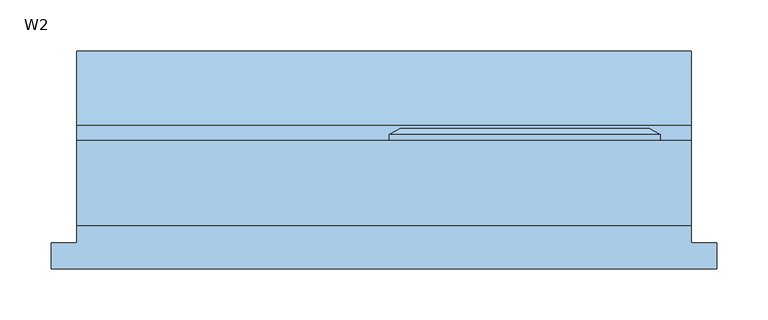
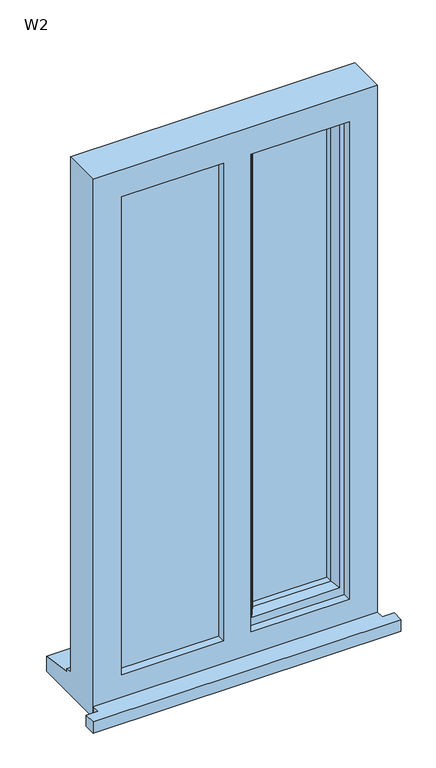
"""IFC4 building model written with IfcOpenShell, lengths in millimetres: window geometry, W2."""

from ifc_helpers import new_model, si_unit, frame, origin, place, context, project, spatial, polyline, outline, extrude, faceted_brep, source, transform, mapped, element, save


def w2_3d16f0f7(model_context):
    return source(origin(), model_context, "Body", "SolidModel", [
        extrude(outline(polyline([(-610.0, -91.5434322), (-610.0, -66.5434322), (-585.0, -66.5434322), (-585.0, -49.5434322), (15.0, -49.5434322), (15.0, -66.5434322), (40.0, -66.5434322), (40.0, -91.5434322), (-610.0, -91.5434322)])), frame((0.0, 0.0, 1200.0), z_axis=(0.0, 0.0, 1.0), x_axis=(1.0, 0.0, 0.0)), (0.0, 0.0, 1.0), 25.0),
        faceted_brep([(-280.0, 33.4565678, 2370.0), (-280.0, 39.2300705, 2370.0), (-280.0, 39.2300705, 1253.0), (-280.0, 33.4565678, 1253.0), (-270.0, -31.5434322, 2360.0), (-270.0, 33.4565678, 2360.0), (-270.0, 33.4565678, 1263.0), (-270.0, -31.5434322, 1263.0), (-230.0, -17.0505323, 2320.0), (-240.1480377, -31.5434322, 2330.1480377), (-240.1480377, -31.5434322, 1292.8519623), (-230.0, -17.0505323, 1303.0), (-230.0, -2.5434322, 2320.0), (-230.0, -2.5434322, 1303.0), (-240.0, 21.4565678, 2330.0), (-240.0, -2.5434322, 2330.0), (-240.0, -2.5434322, 1293.0), (-240.0, 21.4565678, 1293.0), (-230.0, 39.2300705, 2320.0), (-230.0, 21.4565678, 2320.0), (-230.0, 21.4565678, 1303.0), (-230.0, 39.2300705, 1303.0), (-247.4457548, 45.0035732, 2337.4457548), (-247.4457548, 45.0035732, 1285.5542452), (-269.2153903, 45.0035732, 2359.2153903), (-269.2153903, 45.0035732, 1263.7846097), (-15.0, 39.2300705, 1253.0), (-15.0, 33.4565678, 1253.0), (-25.0, 33.4565678, 1263.0), (-25.0, -31.5434322, 1263.0), (-54.8519623, -31.5434322, 1292.8519623), (-65.0, -17.0505323, 1303.0), (-65.0, -2.5434322, 1303.0), (-55.0, -2.5434322, 1293.0), (-55.0, 21.4565678, 1293.0), (-65.0, 21.4565678, 1303.0), (-65.0, 39.2300705, 1303.0), (-47.5542452, 45.0035732, 1285.5542452), (-25.7846097, 45.0035732, 1263.7846097), (-15.0, 39.2300705, 2370.0), (-15.0, 33.4565678, 2370.0), (-25.0, 33.4565678, 2360.0), (-25.0, -31.5434322, 2360.0), (-54.8519623, -31.5434322, 2330.1480377), (-65.0, -17.0505323, 2320.0), (-65.0, -2.5434322, 2320.0), (-55.0, -2.5434322, 2330.0), (-55.0, 21.4565678, 2330.0), (-65.0, 21.4565678, 2320.0), (-65.0, 39.2300705, 2320.0), (-47.5542452, 45.0035732, 2337.4457548), (-25.7846097, 45.0035732, 2359.2153903)], [[[0, 1, 2, 3]], [[4, 5, 6, 7]], [[8, 9, 10, 11]], [[12, 8, 11, 13]], [[14, 15, 16, 17]], [[18, 19, 20, 21]], [[22, 18, 21, 23]], [[1, 24, 25, 2]], [[3, 2, 26, 27]], [[7, 6, 28, 29]], [[11, 10, 30, 31]], [[13, 11, 31, 32]], [[17, 16, 33, 34]], [[21, 20, 35, 36]], [[23, 21, 36, 37]], [[2, 25, 38, 26]], [[27, 26, 39, 40]], [[29, 28, 41, 42]], [[31, 30, 43, 44]], [[32, 31, 44, 45]], [[34, 33, 46, 47]], [[36, 35, 48, 49]], [[37, 36, 49, 50]], [[26, 38, 51, 39]], [[40, 39, 1, 0]], [[3, 27, 40, 0], [5, 41, 28, 6]], [[42, 41, 5, 4]], [[7, 29, 42, 4], [9, 43, 30, 10]], [[44, 43, 9, 8]], [[45, 44, 8, 12]], [[15, 46, 33, 16], [13, 32, 45, 12]], [[47, 46, 15, 14]], [[17, 34, 47, 14], [19, 48, 35, 20]], [[49, 48, 19, 18]], [[50, 49, 18, 22]], [[24, 51, 38, 25], [23, 37, 50, 22]], [[39, 51, 24, 1]]]),
        extrude(outline(polyline([(2340.0, -310.0), (2360.0, -310.0), (2360.0, -545.0), (1263.0, -545.0), (1263.0, -310.0), (1283.0, -310.0), (1283.0, -525.0), (2340.0, -525.0), (2340.0, -310.0)])), frame((0.0, -7.5434322, 0.0), z_axis=(0.0, 1.0, 0.0), x_axis=(0.0, 0.0, 1.0)), (0.0, 0.0, 1.0), 41.0),
        faceted_brep([(15.0, -49.5434322, 2400.0), (-585.0, -49.5434322, 2400.0), (-585.0, -49.5434322, 1200.0), (15.0, -49.5434322, 1200.0), (-45.0, -49.5434322, 2340.0), (-45.0, -49.5434322, 1275.0), (-252.0, -49.5434322, 1275.0), (-252.0, -49.5434322, 2340.0), (-310.0, -49.5434322, 2340.0), (-310.0, -49.5434322, 1275.0), (-525.0, -49.5434322, 1275.0), (-525.0, -49.5434322, 2340.0), (-585.0, 33.4565678, 2400.0), (-585.0, 33.4565678, 1251.0), (-585.0, 48.4565678, 1249.68767), (-585.0, 48.4565678, 1244.7449676), (-585.0, 120.9565678, 1233.8088847), (-585.0, 120.9565678, 1200.0), (15.0, 33.4565678, 2400.0), (15.0, 33.4565678, 1251.0), (-545.0, 33.4565678, 2360.0), (-545.0, 33.4565678, 1263.0), (-310.0, 33.4565678, 1263.0), (-310.0, 33.4565678, 2360.0), (-270.0, 33.4565678, 2360.0), (-270.0, 33.4565678, 1263.0), (-25.0, 33.4565678, 1263.0), (-25.0, 33.4565678, 2360.0), (-545.0, -31.5434322, 2360.0), (-545.0, -31.5434322, 1263.0), (-300.0, -31.5434322, 2360.0), (-300.0, -31.5434322, 1263.0), (-310.0, -31.5434322, 2340.0), (-525.0, -31.5434322, 2340.0), (-525.0, -31.5434322, 1275.0), (-310.0, -31.5434322, 1275.0), (-270.0, -31.5434322, 2360.0), (-25.0, -31.5434322, 2360.0), (-25.0, -31.5434322, 1263.0), (-270.0, -31.5434322, 1263.0), (-45.0, -31.5434322, 2340.0), (-252.0, -31.5434322, 2340.0), (-252.0, -31.5434322, 1275.0), (-45.0, -31.5434322, 1275.0), (-310.0, -7.5434322, 2360.0), (-300.0, -7.5434322, 2360.0), (15.0, 120.9565678, 1200.0), (15.0, 120.9565678, 1233.8088847), (15.0, 48.4565678, 1244.7449676), (15.0, 48.4565678, 1249.68767), (-300.0, -7.5434322, 1263.0), (-310.0, -7.5434322, 1263.0)], [[[0, 1, 2, 3], [4, 5, 6, 7], [8, 9, 10, 11]], [[2, 1, 12, 13, 14, 15, 16, 17]], [[13, 12, 18, 19], [20, 21, 22, 23], [24, 25, 26, 27]], [[21, 20, 28, 29]], [[28, 30, 31, 29], [32, 33, 34, 35]], [[36, 37, 38, 39], [40, 41, 42, 43]], [[33, 11, 10, 34]], [[1, 0, 18, 12]], [[28, 20, 23, 44, 45, 30]], [[27, 37, 36, 24]], [[11, 33, 32, 8]], [[40, 4, 7, 41]], [[19, 18, 0, 3, 46, 47, 48, 49]], [[27, 26, 38, 37]], [[4, 40, 43, 5]], [[45, 50, 31, 30]], [[50, 45, 44, 51]], [[51, 44, 23, 22]], [[25, 24, 36, 39]], [[41, 7, 6, 42]], [[8, 32, 35, 9]], [[46, 3, 2, 17]], [[47, 46, 17, 16]], [[48, 47, 16, 15]], [[49, 48, 15, 14]], [[19, 49, 14, 13]], [[22, 21, 29, 31, 50, 51]], [[26, 25, 39, 38]], [[6, 5, 43, 42]], [[35, 34, 10, 9]]]),
        extrude(outline(polyline([(-545.0, -7.5434322), (-300.0, -7.5434322), (-300.0, -31.5434322), (-545.0, -31.5434322), (-545.0, -7.5434322)])), frame((0.0, 0.0, 1263.0), z_axis=(0.0, 0.0, 1.0), x_axis=(1.0, 0.0, 0.0)), (0.0, 0.0, 1.0), 1097.0),
        extrude(outline(polyline([(-55.0, -2.5434322), (-240.0, -2.5434322), (-240.0, 21.4565678), (-55.0, 21.4565678), (-55.0, -2.5434322)])), frame((0.0, 0.0, 1293.0), z_axis=(0.0, 0.0, 1.0), x_axis=(1.0, 0.0, 0.0)), (0.0, 0.0, 1.0), 1037.0),
    ])


if __name__ == "__main__":
    model = new_model("IFC4")
    model_context = context("Model", 3, world=origin())
    ifc_project = project(units=[si_unit("LENGTHUNIT", "METRE", prefix="MILLI")], contexts=[model_context])
    site = spatial("IfcSite", under=ifc_project)
    building = spatial("IfcBuilding", under=site)
    placement = place(None, origin())
    w2_shape = w2_3d16f0f7(model_context)
    element("IfcWindow", 1, ObjectType="W2", at=placement, inside=building, context=model_context, shape_type="MappedRepresentation", body=[
        mapped(w2_shape, transform((0.0, 0.0, 0.0), x_axis=(1.0, 0.0, 0.0), y_axis=(0.0, 1.0, 0.0), z_axis=(0.0, 0.0, 1.0))),
    ])
    save(model, "model.ifc")

# Revit data of these elements
# Type "W2"
#   Type Mark = "42"
#   Operation = "DoublePanelVertical"
#   Manufacturer = "Revit"
#   Wrap Layers (Ext) from Ext = 102.5 mm
#   Wrap Layers (Int) from Ext = 177.5 mm
#   Window Board Projection = 25 mm
#   Window Board Extension = 25 mm
#   Rough Width = 600 mm
#   Rough Height = 1200 mm
#   Height = 1200 mm
#   Width = 600 mm
#   Glazing Thickness = 24 mm
#   FrameOffset - External = 50 mm
#   Frame Depth = 65 mm
#   Default Head Height = 2400 mm
#   Cill Depth = 87.5 mm
#   Cavity Closer Width = 50 mm
#   Cavity Closer Offset from Ext = 102.5 mm
#   Cavity Closer Depth = 85 mm
#   Vis - Cavity Closers = yes
#   Material Trim = Window Frame
#   Material Glass = Glass
#   Material Frame = Window Frame
#   Wall Closure = (empty or 0)
# Element 1 (IfcWindow, "W2")
#   Materials on its faces: "Window Frame", "Glass"
# Materials
#   "Window Frame": colour RGB 249 249 249, transparency 0
#   "Glass": class "Glass", colour RGB 245 245 243, transparency 1, Description = "Soda Lime Glass", Cost = 0
